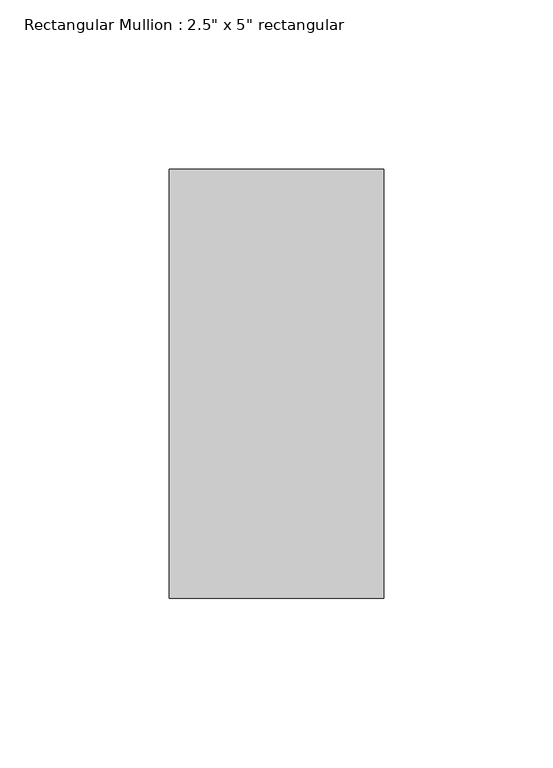
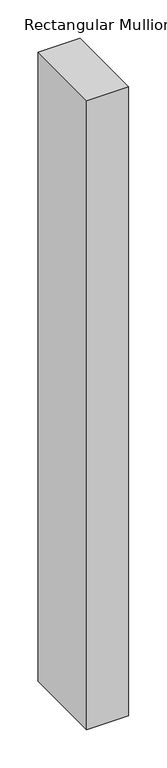
"""IFC4 building model written with IfcOpenShell, lengths in millimetres: member geometry."""

from ifc_helpers import new_model, si_unit, frame, origin, place, context, project, spatial, polyline, outline, extrude, source, transform, mapped, element, save


def member_7fa3b085(model_context):
    return source(origin(), model_context, "Body", "SweptSolid", [
        extrude(outline(polyline([(31.75, 63.5), (31.75, -63.5), (-31.75, -63.5), (-31.75, 63.5), (31.75, 63.5)])), frame((0.0, 0.0, -1003.3), z_axis=(0.0, 0.0, 1.0), x_axis=(1.0, 0.0, 0.0)), (0.0, 0.0, 1.0), 1003.3),
    ])


if __name__ == "__main__":
    model = new_model("IFC4")
    model_context = context("Model", 3, world=origin())
    ifc_project = project(units=[si_unit("LENGTHUNIT", "METRE", prefix="MILLI")], contexts=[model_context])
    site = spatial("IfcSite", under=ifc_project)
    building = spatial("IfcBuilding", under=site)
    placement = place(None, origin())
    member_shape = member_7fa3b085(model_context)
    element("IfcMember", 1, ObjectType="Rectangular Mullion : 2.5\" x 5\" rectangular", at=placement, inside=building, context=model_context, shape_type="MappedRepresentation", body=[
        mapped(member_shape, transform((0.0, 0.0, 0.0), x_axis=(1.0, 0.0, 0.0), y_axis=(0.0, 1.0, 0.0), z_axis=(0.0, 0.0, 1.0))),
    ])
    save(model, "model.ifc")

# Revit data of these elements
# Type "Rectangular Mullion : 2.5\" x 5\" rectangular"
#   built-in parameter 1007304 = 0.416667 (stored number, unit not read)
#   built-in parameter 1007301 = 0.104167 (stored number, unit not read)
#   built-in parameter 1007300 = 0.104167 (stored number, unit not read)
# Element 1 (IfcMember, "Rectangular Mullion : 2.5\" x 5\" rectangular")
#   Materials on its faces: "Aluminum"
# Materials
#   "Aluminum": class "Metal", colour RGB 247 247 247, transparency 0, Description = "Aluminum 6061", Cost = 0
